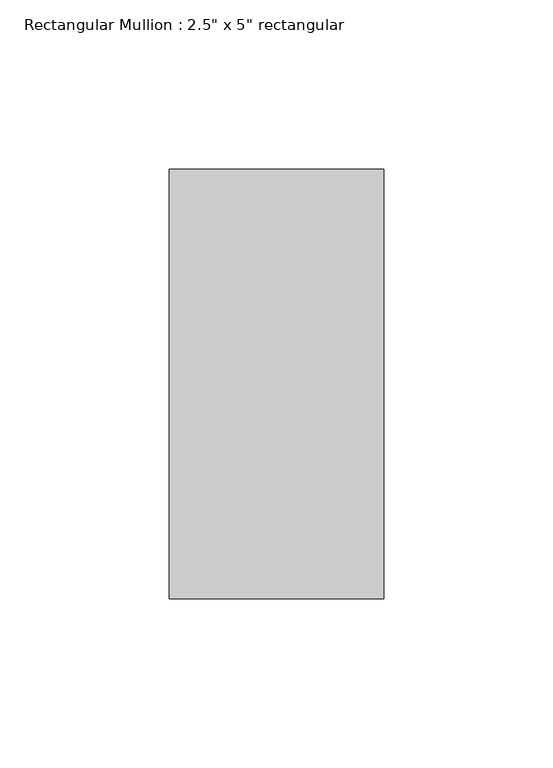
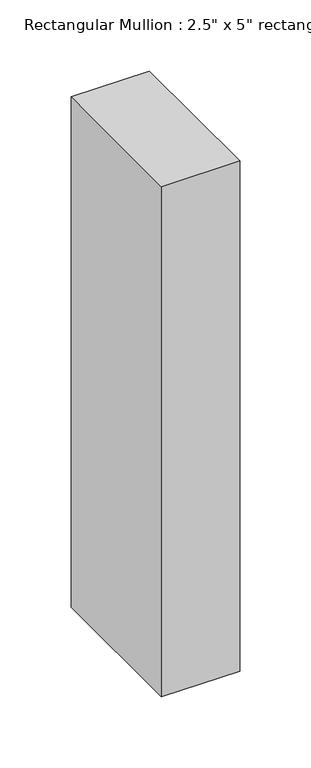
"""IFC4 building model written with IfcOpenShell, lengths in millimetres: member geometry."""

from ifc_helpers import new_model, si_unit, frame, origin, place, context, project, spatial, polyline, outline, extrude, source, transform, mapped, element, save


def member_6fb4a552(model_context):
    return source(origin(), model_context, "Body", "SweptSolid", [
        extrude(outline(polyline([(0.0, 63.5), (0.0, -63.5), (-63.5, -63.5), (-63.5, 63.5), (0.0, 63.5)])), frame((0.0, 0.0, -438.15), z_axis=(0.0, 0.0, 1.0), x_axis=(1.0, 0.0, 0.0)), (0.0, 0.0, 1.0), 438.15),
    ])


if __name__ == "__main__":
    model = new_model("IFC4")
    model_context = context("Model", 3, world=origin())
    ifc_project = project(units=[si_unit("LENGTHUNIT", "METRE", prefix="MILLI")], contexts=[model_context])
    site = spatial("IfcSite", under=ifc_project)
    building = spatial("IfcBuilding", under=site)
    placement = place(None, origin())
    member_shape = member_6fb4a552(model_context)
    element("IfcMember", 1, ObjectType="Rectangular Mullion : 2.5\" x 5\" rectangular", at=placement, inside=building, context=model_context, shape_type="MappedRepresentation", body=[
        mapped(member_shape, transform((0.0, 0.0, 0.0), x_axis=(1.0, 0.0, 0.0), y_axis=(0.0, 1.0, 0.0), z_axis=(0.0, 0.0, 1.0))),
    ])
    save(model, "model.ifc")

# Revit data of these elements
# Type "Rectangular Mullion : 2.5\" x 5\" rectangular"
#   built-in parameter 1007304 = 0.416667 (stored number, unit not read)
#   built-in parameter 1007301 = 0.104167 (stored number, unit not read)
#   built-in parameter 1007300 = 0.104167 (stored number, unit not read)
